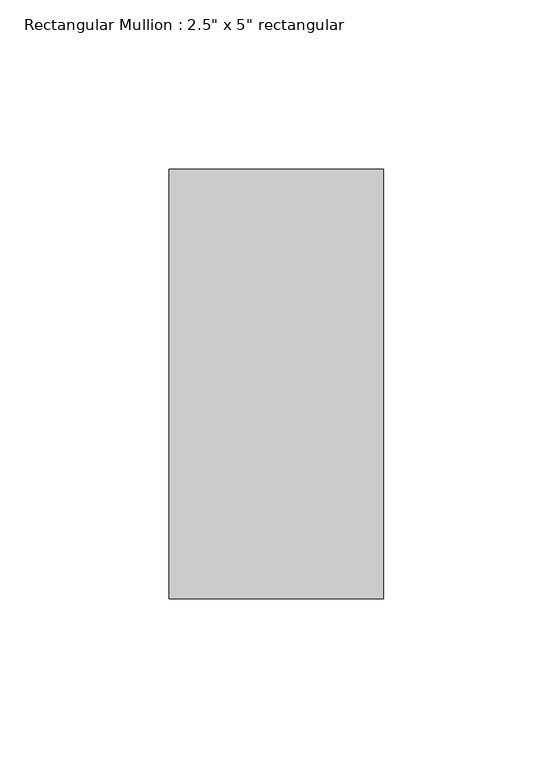
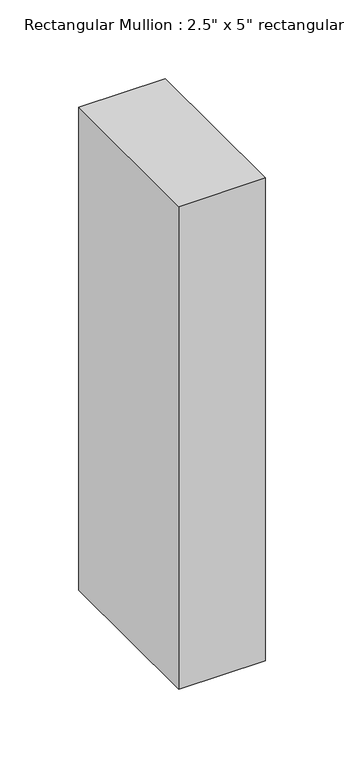
"""IFC4 building model written with IfcOpenShell, lengths in millimetres: member geometry."""

from ifc_helpers import new_model, si_unit, frame, origin, place, context, project, spatial, polyline, outline, extrude, source, transform, mapped, element, save


def member_8d9b4452(model_context):
    return source(origin(), model_context, "Body", "SweptSolid", [
        extrude(outline(polyline([(0.0, 63.5), (0.0, -63.5), (-63.5, -63.5), (-63.5, 63.5), (0.0, 63.5)])), frame((0.0, 0.0, -374.65), z_axis=(0.0, 0.0, 1.0), x_axis=(1.0, 0.0, 0.0)), (0.0, 0.0, 1.0), 374.65),
    ])


if __name__ == "__main__":
    model = new_model("IFC4")
    model_context = context("Model", 3, world=origin())
    ifc_project = project(units=[si_unit("LENGTHUNIT", "METRE", prefix="MILLI")], contexts=[model_context])
    site = spatial("IfcSite", under=ifc_project)
    building = spatial("IfcBuilding", under=site)
    placement = place(None, origin())
    member_shape = member_8d9b4452(model_context)
    element("IfcMember", 1, ObjectType="Rectangular Mullion : 2.5\" x 5\" rectangular", at=placement, inside=building, context=model_context, shape_type="MappedRepresentation", body=[
        mapped(member_shape, transform((0.0, 0.0, 0.0), x_axis=(1.0, 0.0, 0.0), y_axis=(0.0, 1.0, 0.0), z_axis=(0.0, 0.0, 1.0))),
    ])
    save(model, "model.ifc")

# Revit data of these elements
# Type "Rectangular Mullion : 2.5\" x 5\" rectangular"
#   built-in parameter 1007304 = 0.416667 (stored number, unit not read)
#   built-in parameter 1007301 = 0.104167 (stored number, unit not read)
#   built-in parameter 1007300 = 0.104167 (stored number, unit not read)
